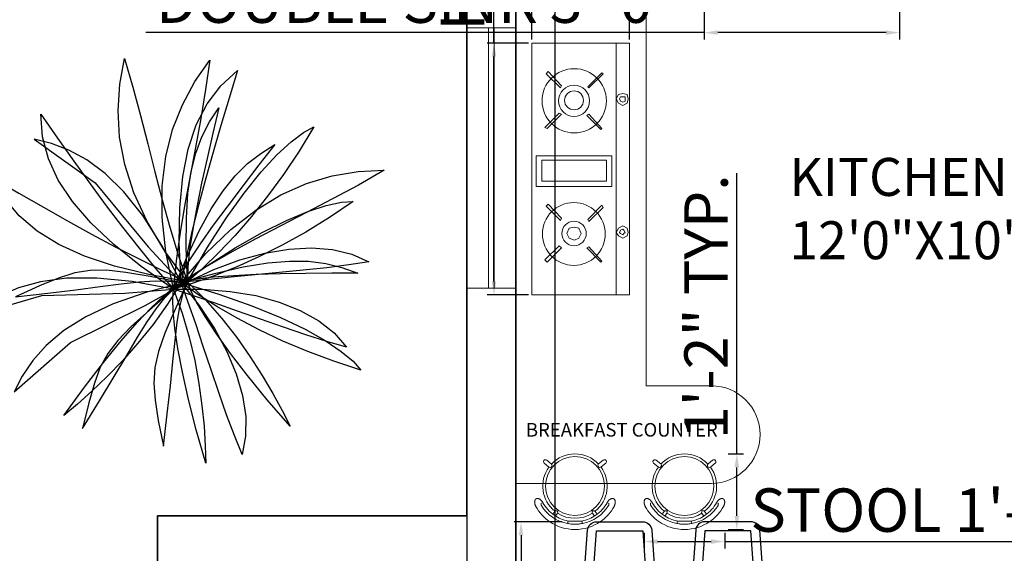
# Model space of a CAD drawing. Units: inches. Extents: x 3394 to 4794, y 965 to 1718.
# Tile 8 of 15: x 3522 to 3704, y 1450 to 1548. Entities that reach past the tile are written whole.
import ezdxf

# ---------------------------------------------------------------- set-up
doc = ezdxf.new("R2010")
doc.units = ezdxf.units.IN
for name, color, linetype, lineweight in [('A-ANNO-DIMS', 2, 'Continuous', 13), ('A-ANNO-TEXT', 7, 'Continuous', 18), ('A-AREA-IDEN', 7, 'Continuous', 18), ('A-EQPM', 8, 'Continuous', 18), ('A-FLOR-CASE', 8, 'Continuous', 18), ('A-GLAZ', 4, 'Continuous', 18), ('A-WALL', 7, 'Continuous', 35), ('CAY', 94, 'Continuous', 13), ('NOITHAT', 21, 'Continuous', 18)]:
    doc.layers.add(name, color=color, linetype=linetype, lineweight=lineweight)
doc.layers.add('DIENHOA', color=3, linetype='Continuous')
doc.layers.add('NOI THAT', color=42, linetype='Continuous')
doc.styles.get("Standard").update_dxf_attribs({"font": 'arial.ttf'})
doc.dimstyles.new('ISO-25', dxfattribs={"dimtxt": 8, "dimasz": 2.5, "dimexe": 1.25, "dimexo": 0.625, "dimtad": 1, "dimlunit": 3, "dimtxsty": 'Standard', "dimcen": 2.5, "dimadec": 0, "dimazin": 0, "dimtfac": 1, "dimtmove": 0, "dimatfit": 3, "dimfxl": 1, "dimarcsym": 0})

# ---------------------------------------------------------------- blocks, each defined once
blk = doc.blocks.new('gas 1')
for points in [[(35.93, -1.87), (35.93, 0), (0, 0), (0, -1.87)], [(8.12, -0.94), (8.44, -1.56), (8.91, -1.87), (9.53, -1.56), (9.84, -0.94), (9.53, -0.31), (8.91, -0.16), (8.44, -0.31)], [(8.59, -0.94), (8.75, -1.25), (8.91, -1.41), (9.22, -1.25), (9.37, -0.94), (9.22, -0.78), (8.91, -0.62), (8.75, -0.78)], [(27.03, -0.94), (27.34, -1.56), (27.97, -1.87), (28.59, -1.56), (28.75, -0.94), (28.59, -0.31), (27.97, -0.16), (27.34, -0.31)], [(27.5, -0.94), (27.65, -1.25), (27.97, -1.41), (28.28, -1.25), (28.28, -0.94), (28.28, -0.62), (27.97, -0.62), (27.65, -0.62)], [(19.84, -13.28), (15.47, -13.28), (15.47, -2.5), (19.84, -2.5)], [(4.84, -3.91), (4.69, -4.06), (6.72, -6.09), (6.87, -5.78)], [(12.81, -3.91), (12.5, -3.75), (10.47, -5.78), (10.78, -5.94)], [(19.22, -12.5), (16.25, -12.5), (16.25, -3.28), (19.22, -3.28)], [(23.75, -3.91), (23.59, -4.06), (25.62, -6.09), (25.78, -5.78)], [(31.71, -3.91), (31.56, -3.75), (29.53, -5.78), (29.68, -5.94)], [(7.81, -7.81), (8.12, -8.59), (8.75, -8.91), (9.53, -8.59), (9.69, -7.81), (9.53, -7.19), (8.75, -6.87), (8.12, -7.19)], [(7.03, -10), (6.72, -9.69), (4.69, -11.72), (5, -12.03)], [(12.97, -11.56), (10.94, -9.69), (10.62, -9.84), (12.65, -11.87)], [(23.75, -11.72), (23.9, -12.03), (25.93, -10), (25.78, -9.69)], [(31.87, -11.56), (29.84, -9.69), (29.53, -9.84), (31.56, -11.87)]]:
    blk.add_lwpolyline(points, close=True)
blk.add_lwpolyline([(35.93, -1.87), (35.93, -13.9), (0, -13.9), (0, -1.87)])
for centre, radius in [((8.7, -7.92), 4.48), ((27.7, -7.86), 4.58), ((8.77, -7.89), 1.74), ((27.69, -7.89), 2.22), ((27.76, -7.89), 1.35)]:
    blk.add_circle(centre, radius)
blk = doc.blocks.new('A$C02103572')
at = {"layer": 'NOI THAT'}
for p, q in [((450, 1200), (450, 0)), ((1200, 1200), (450, 1200)), ((1200, 0), (1200, 1200)), ((350, 750.1), (350, 1049.9)), ((1300, 750.1), (1300, 1049.9)), ((350, 449.9), (350, 150.1)), ((1300, 449.9), (1300, 150.1)), ((450, 0), (1200, 0))]:
    blk.add_line(p, q, dxfattribs=at)
for points in [[(350, 1100), (46.9, 1077.9, 0.396047), (0, 1028), (0, 772, 0.396047), (46.9, 722.1), (346.4, 700.3)], [(1300, 1100), (1603.1, 1077.9, -0.396047), (1650, 1028), (1650, 772, -0.396047), (1603.1, 722.1), (1303.6, 700.3)], [(350, 100), (46.9, 122.1, -0.396047), (0, 172), (0, 428, -0.396047), (46.9, 477.9), (346.4, 499.7)], [(1300, 100), (1603.1, 122.1, 0.396047), (1650, 172), (1650, 428, 0.396047), (1603.1, 477.9), (1303.6, 499.7)]]:
    blk.add_lwpolyline(points, format="xyb", dxfattribs=at)
for points in [[(353.6, 1050.1), (50, 1028), (50, 772), (350, 750.1)], [(1296.4, 1050.1), (1600, 1028), (1600, 772), (1300, 750.1)], [(353.6, 149.9), (50, 172), (50, 428), (350, 449.9)], [(1296.4, 149.9), (1600, 172), (1600, 428), (1300, 449.9)]]:
    blk.add_lwpolyline(points, dxfattribs=at)
for centre, start, end in [((351.8, 1075.1), 274.1643, 94.1643), ((1298.2, 1075.1), 85.8357, 265.8357), ((348.2, 725.2), 265.8357, 85.8357), ((1301.8, 725.2), 94.1643, 274.1643), ((348.2, 474.8), 274.1643, 94.1643), ((1301.8, 474.8), 85.8357, 265.8357), ((351.8, 124.9), 265.8357, 85.8357), ((1298.2, 124.9), 94.1643, 274.1643)]:
    blk.add_arc(centre, 25, start, end, dxfattribs=at)
blk = doc.blocks.new('SILLA 01')
for p, q in [((-0.1216, 0.2388), (-0.1198, 0.2397)), ((-0.1198, 0.2397), (-0.118, 0.2405)), ((-0.118, 0.2405), (-0.1161, 0.2412)), ((-0.1161, 0.2412), (-0.1143, 0.2419)), ((-0.1143, 0.2419), (-0.1124, 0.2426)), ((-0.1124, 0.2426), (-0.1104, 0.2431)), ((-0.1104, 0.2431), (-0.1085, 0.2437)), ((-0.1085, 0.2437), (-0.1069, 0.244)), ((-0.1069, 0.244), (-0.1053, 0.2444)), ((-0.1053, 0.2444), (-0.1037, 0.2446)), ((-0.1037, 0.2446), (-0.102, 0.2448)), ((-0.102, 0.2448), (-0.1004, 0.2449)), ((-0.1004, 0.2449), (-0.0987, 0.245)), ((-0.0987, 0.245), (-0.0971, 0.245)), ((-0.0971, 0.245), (-0.0954, 0.2449)), ((-0.0954, 0.2449), (-0.0939, 0.2448)), ((-0.0939, 0.2448), (-0.0924, 0.2446)), ((-0.0924, 0.2446), (-0.0908, 0.2443)), ((-0.0908, 0.2443), (-0.0893, 0.2439)), ((-0.0893, 0.2439), (-0.0878, 0.2435)), ((-0.0878, 0.2435), (-0.0864, 0.243)), ((-0.0864, 0.243), (-0.0849, 0.2423)), ((-0.0849, 0.2423), (-0.0836, 0.2417)), ((-0.0836, 0.2417), (-0.0826, 0.2411)), ((-0.0826, 0.2411), (-0.0817, 0.2405)), ((-0.0817, 0.2405), (-0.0808, 0.2398)), ((-0.0808, 0.2398), (-0.08, 0.239)), ((-0.1968, 0.1793), (-0.186, 0.1909)), ((-0.186, 0.1909), (-0.1746, 0.2017)), ((-0.1746, 0.2017), (-0.1626, 0.2119)), ((-0.1626, 0.2119), (-0.1501, 0.2213)), ((-0.1571, 0.1744), (-0.1381, 0.1904)), ((-0.1501, 0.2213), (-0.137, 0.23)), ((-0.1381, 0.1904), (-0.1176, 0.2043)), ((-0.137, 0.23), (-0.1234, 0.2379)), ((-0.1334, 0.1739), (-0.123, 0.1816)), ((-0.1234, 0.2379), (-0.1216, 0.2388)), ((-0.123, 0.1816), (-0.1123, 0.1887)), ((-0.1176, 0.2043), (-0.1159, 0.2052)), ((-0.1159, 0.2052), (-0.1142, 0.2058)), ((-0.1142, 0.2058), (-0.1123, 0.2062)), ((-0.1123, 0.2062), (-0.1104, 0.2063)), ((-0.1123, 0.1887), (-0.1012, 0.1952)), ((-0.1104, 0.2063), (-0.1086, 0.2062)), ((-0.1086, 0.2062), (-0.1067, 0.2058)), ((-0.1067, 0.2058), (-0.105, 0.2051)), ((-0.105, 0.2051), (-0.1033, 0.2042)), ((-0.0994, 0.1962), (-0.1012, 0.1952)), ((-0.0977, 0.1972), (-0.0994, 0.1962)), ((-0.096, 0.1983), (-0.0977, 0.1972)), ((-0.0943, 0.1994), (-0.096, 0.1983)), ((-0.0927, 0.2006), (-0.0943, 0.1994)), ((-0.0911, 0.2019), (-0.0927, 0.2006)), ((-0.0896, 0.2031), (-0.0911, 0.2019)), ((-0.0881, 0.2045), (-0.0896, 0.2031)), ((-0.0869, 0.2056), (-0.0881, 0.2045)), ((-0.0857, 0.2068), (-0.0869, 0.2056)), ((-0.0846, 0.208), (-0.0857, 0.2068)), ((-0.0835, 0.2093), (-0.0846, 0.208)), ((-0.0825, 0.2106), (-0.0835, 0.2093)), ((-0.0815, 0.212), (-0.0825, 0.2106)), ((-0.0806, 0.2133), (-0.0815, 0.212)), ((-0.0797, 0.2148), (-0.0806, 0.2133)), ((-0.08, 0.239), (-0.0792, 0.2382)), ((-0.0789, 0.2161), (-0.0797, 0.2148)), ((-0.0792, 0.2382), (-0.0785, 0.2373)), ((-0.0782, 0.2176), (-0.0789, 0.2161)), ((-0.0785, 0.2373), (-0.0779, 0.2364)), ((-0.0776, 0.219), (-0.0782, 0.2176)), ((-0.0779, 0.2364), (-0.0773, 0.2354)), ((-0.0771, 0.2205), (-0.0776, 0.219)), ((-0.0773, 0.2354), (-0.0769, 0.2344)), ((-0.0766, 0.222), (-0.0771, 0.2205)), ((-0.0769, 0.2344), (-0.0764, 0.2333)), ((-0.0762, 0.2235), (-0.0766, 0.222)), ((-0.0764, 0.2333), (-0.0761, 0.2322)), ((-0.0759, 0.2251), (-0.0762, 0.2235)), ((-0.0761, 0.2322), (-0.0759, 0.2311)), ((-0.0759, 0.2311), (-0.0757, 0.23)), ((-0.0757, 0.2266), (-0.0759, 0.2251)), ((-0.0757, 0.23), (-0.0756, 0.2289)), ((-0.0756, 0.2278), (-0.0757, 0.2266)), ((-0.0756, 0.2289), (-0.0756, 0.2278)), ((0.1165, 0.1601), (0.1387, 0.1871)), ((0.1387, 0.1871), (0.1425, 0.1901)), ((0.1425, 0.1901), (0.1471, 0.1915)), ((0.1471, 0.1915), (0.1519, 0.191)), ((0.1519, 0.191), (0.1561, 0.1886)), ((0.1561, 0.1886), (0.1592, 0.1848)), ((0.1592, 0.1848), (0.1605, 0.1801)), ((0.1605, 0.1801), (0.16, 0.1752)), ((-0.2367, 0.1191), (-0.2271, 0.1372)), ((-0.2271, 0.1372), (-0.2162, 0.1544)), ((-0.2162, 0.1544), (-0.2068, 0.1672)), ((-0.2068, 0.1672), (-0.1968, 0.1793)), ((-0.2028, 0.1156), (-0.1896, 0.1368)), ((-0.1896, 0.1368), (-0.1744, 0.1565)), ((-0.1835, 0.1171), (-0.1773, 0.1267)), ((-0.1773, 0.1267), (-0.1696, 0.1372)), ((-0.1744, 0.1565), (-0.1571, 0.1744)), ((-0.1538, 0.1223), (-0.1714, 0.1348)), ((-0.1696, 0.1372), (-0.1614, 0.1472)), ((-0.1614, 0.1472), (-0.1525, 0.1566)), ((-0.1538, 0.1223), (-0.1511, 0.1194)), ((-0.1525, 0.1566), (-0.1432, 0.1655)), ((-0.1432, 0.1655), (-0.1334, 0.1739)), ((0.1136, 0.1509), (0.1141, 0.1558)), ((0.115, 0.1462), (0.1136, 0.1509)), ((0.1141, 0.1558), (0.1165, 0.1601)), ((0.118, 0.1423), (0.115, 0.1462)), ((0.1222, 0.14), (0.118, 0.1423)), ((0.127, 0.1394), (0.1222, 0.14)), ((0.1317, 0.1408), (0.127, 0.1394)), ((0.1354, 0.1439), (0.1317, 0.1408)), ((0.1577, 0.1709), (0.1354, 0.1439)), ((0.16, 0.1752), (0.1577, 0.1709)), ((-0.2609, 0.041), (-0.2571, 0.0611)), ((-0.2571, 0.0611), (-0.2518, 0.081)), ((-0.2518, 0.081), (-0.245, 0.1003)), ((-0.245, 0.1003), (-0.2367, 0.1191)), ((-0.2281, 0.0453), (-0.2221, 0.0696)), ((-0.2221, 0.0696), (-0.2136, 0.0931)), ((-0.2136, 0.0931), (-0.2028, 0.1156)), ((-0.2101, 0.0535), (-0.207, 0.0646)), ((-0.207, 0.0646), (-0.2034, 0.0756)), ((-0.2034, 0.0756), (-0.1993, 0.0864)), ((-0.1993, 0.0864), (-0.1945, 0.0969)), ((-0.1945, 0.0969), (-0.1893, 0.1071)), ((-0.1893, 0.1071), (-0.1835, 0.1171)), ((-0.1828, 0.1184), (-0.1651, 0.1058)), ((-0.1616, 0.1042), (-0.1651, 0.1058)), ((-0.1577, 0.1041), (-0.1616, 0.1042)), ((-0.1541, 0.1055), (-0.1577, 0.1041)), ((-0.1513, 0.1083), (-0.1541, 0.1055)), ((-0.1498, 0.1118), (-0.1513, 0.1083)), ((-0.1511, 0.1194), (-0.1497, 0.1158)), ((-0.1497, 0.1158), (-0.1498, 0.1118)), ((-0.264, 0), (-0.2632, 0.0205)), ((-0.2632, -0.0205), (-0.264, 0)), ((-0.2632, 0.0205), (-0.2609, 0.041)), ((-0.2318, 0), (-0.2317, 0.0057)), ((-0.2317, -0.0057), (-0.2318, 0)), ((-0.2317, 0.0057), (-0.2315, 0.0114)), ((-0.2315, 0.0114), (-0.2312, 0.017)), ((-0.2312, 0.017), (-0.2307, 0.0227)), ((-0.2307, 0.0227), (-0.2301, 0.0283)), ((-0.2301, 0.0283), (-0.2294, 0.034)), ((-0.2294, 0.034), (-0.2285, 0.0396)), ((-0.2285, 0.0396), (-0.2275, 0.0452)), ((-0.2125, 0.0422), (-0.2275, 0.0452)), ((-0.2125, 0.0422), (-0.2101, 0.0535)), ((-0.2125, 0.0422), (-0.2125, -0.0422)), ((-0.2609, -0.041), (-0.2632, -0.0205)), ((-0.2571, -0.0611), (-0.2609, -0.041)), ((-0.2315, -0.0114), (-0.2317, -0.0057)), ((-0.2312, -0.017), (-0.2315, -0.0114)), ((-0.2307, -0.0227), (-0.2312, -0.017)), ((-0.2301, -0.0283), (-0.2307, -0.0227)), ((-0.2294, -0.034), (-0.2301, -0.0283)), ((-0.2285, -0.0396), (-0.2294, -0.034)), ((-0.2275, -0.0452), (-0.2285, -0.0396)), ((-0.2221, -0.0696), (-0.2281, -0.0453)), ((-0.2125, -0.0422), (-0.2275, -0.0452)), ((-0.2101, -0.0535), (-0.2125, -0.0422)), ((-0.207, -0.0646), (-0.2101, -0.0535)), ((-0.2518, -0.081), (-0.2571, -0.0611)), ((-0.245, -0.1003), (-0.2518, -0.081)), ((-0.2367, -0.1191), (-0.245, -0.1003)), ((-0.2271, -0.1372), (-0.2367, -0.1191)), ((-0.2136, -0.0931), (-0.2221, -0.0696)), ((-0.2028, -0.1156), (-0.2136, -0.0931)), ((-0.2034, -0.0756), (-0.207, -0.0646)), ((-0.1993, -0.0864), (-0.2034, -0.0756)), ((-0.1896, -0.1368), (-0.2028, -0.1156)), ((-0.1945, -0.0969), (-0.1993, -0.0864)), ((-0.1893, -0.1071), (-0.1945, -0.0969)), ((-0.1835, -0.1171), (-0.1893, -0.1071)), ((-0.1773, -0.1267), (-0.1835, -0.1171)), ((-0.1828, -0.1184), (-0.1651, -0.1058)), ((-0.1651, -0.1058), (-0.1616, -0.1042)), ((-0.1616, -0.1042), (-0.1577, -0.1041)), ((-0.1577, -0.1041), (-0.1541, -0.1055)), ((-0.1541, -0.1055), (-0.1513, -0.1083)), ((-0.1511, -0.1194), (-0.1538, -0.1223)), ((-0.1513, -0.1083), (-0.1498, -0.1118)), ((-0.1497, -0.1158), (-0.1511, -0.1194)), ((-0.1498, -0.1118), (-0.1497, -0.1158)), ((-0.2162, -0.1544), (-0.2271, -0.1372)), ((-0.2068, -0.1672), (-0.2162, -0.1544)), ((-0.1968, -0.1793), (-0.2068, -0.1672)), ((-0.186, -0.1909), (-0.1968, -0.1793)), ((-0.1744, -0.1565), (-0.1896, -0.1368)), ((-0.1696, -0.1372), (-0.1773, -0.1267)), ((-0.1571, -0.1744), (-0.1744, -0.1565)), ((-0.1538, -0.1223), (-0.1714, -0.1348)), ((-0.1614, -0.1472), (-0.1696, -0.1372)), ((-0.1525, -0.1566), (-0.1614, -0.1472)), ((-0.1381, -0.1904), (-0.1571, -0.1744)), ((-0.1432, -0.1655), (-0.1525, -0.1566)), ((-0.1334, -0.1739), (-0.1432, -0.1655)), ((-0.123, -0.1816), (-0.1334, -0.1739)), ((0.1136, -0.1509), (0.115, -0.1462)), ((0.1141, -0.1558), (0.1136, -0.1509)), ((0.1165, -0.1601), (0.1141, -0.1558)), ((0.115, -0.1462), (0.118, -0.1423)), ((0.1165, -0.1601), (0.1387, -0.1871)), ((0.118, -0.1423), (0.1222, -0.14)), ((0.1222, -0.14), (0.127, -0.1394)), ((0.127, -0.1394), (0.1317, -0.1408)), ((0.1317, -0.1408), (0.1354, -0.1439)), ((0.1577, -0.1709), (0.1354, -0.1439)), ((0.1577, -0.1709), (0.16, -0.1752)), ((0.16, -0.1752), (0.1605, -0.1801)), ((-0.1746, -0.2017), (-0.186, -0.1909)), ((-0.1626, -0.2119), (-0.1746, -0.2017)), ((-0.1501, -0.2213), (-0.1626, -0.2119)), ((-0.137, -0.23), (-0.1501, -0.2213)), ((-0.1176, -0.2043), (-0.1381, -0.1904)), ((-0.1234, -0.2379), (-0.137, -0.23)), ((-0.1216, -0.2388), (-0.1234, -0.2379)), ((-0.1123, -0.1887), (-0.123, -0.1816)), ((-0.1198, -0.2397), (-0.1216, -0.2388)), ((-0.1159, -0.2052), (-0.1176, -0.2043)), ((-0.1142, -0.2058), (-0.1159, -0.2052)), ((-0.1123, -0.2062), (-0.1142, -0.2058)), ((-0.1012, -0.1952), (-0.1123, -0.1887)), ((-0.1104, -0.2063), (-0.1123, -0.2062)), ((-0.1086, -0.2062), (-0.1104, -0.2063)), ((-0.1067, -0.2058), (-0.1086, -0.2062)), ((-0.105, -0.2051), (-0.1067, -0.2058)), ((-0.1033, -0.2042), (-0.105, -0.2051)), ((-0.1012, -0.1952), (-0.0994, -0.1962)), ((-0.0994, -0.1962), (-0.0977, -0.1972)), ((-0.0977, -0.1972), (-0.096, -0.1983)), ((-0.096, -0.1983), (-0.0943, -0.1994)), ((-0.0943, -0.1994), (-0.0927, -0.2006)), ((-0.0927, -0.2006), (-0.0911, -0.2019)), ((-0.0911, -0.2019), (-0.0896, -0.2031)), ((-0.0896, -0.2031), (-0.0881, -0.2045)), ((-0.0881, -0.2045), (-0.0869, -0.2056)), ((-0.0869, -0.2056), (-0.0857, -0.2068)), ((-0.0857, -0.2068), (-0.0846, -0.208)), ((-0.0846, -0.208), (-0.0835, -0.2093)), ((-0.0835, -0.2093), (-0.0825, -0.2106)), ((-0.0825, -0.2106), (-0.0815, -0.212)), ((-0.0815, -0.212), (-0.0806, -0.2133)), ((-0.08, -0.239), (-0.0808, -0.2398)), ((-0.0806, -0.2133), (-0.0797, -0.2148)), ((-0.0792, -0.2382), (-0.08, -0.239)), ((-0.0797, -0.2148), (-0.0789, -0.2161)), ((-0.0785, -0.2373), (-0.0792, -0.2382)), ((-0.0789, -0.2161), (-0.0782, -0.2176)), ((-0.0779, -0.2364), (-0.0785, -0.2373)), ((-0.0782, -0.2176), (-0.0776, -0.219)), ((-0.0773, -0.2354), (-0.0779, -0.2364)), ((-0.0776, -0.219), (-0.0771, -0.2205)), ((-0.0769, -0.2344), (-0.0773, -0.2354)), ((-0.0771, -0.2205), (-0.0766, -0.222)), ((-0.0764, -0.2333), (-0.0769, -0.2344)), ((-0.0766, -0.222), (-0.0762, -0.2235)), ((-0.0761, -0.2322), (-0.0764, -0.2333)), ((-0.0762, -0.2235), (-0.0759, -0.2251)), ((-0.0759, -0.2311), (-0.0761, -0.2322)), ((-0.0759, -0.2251), (-0.0757, -0.2266)), ((-0.0757, -0.23), (-0.0759, -0.2311)), ((-0.0757, -0.2266), (-0.0756, -0.2278)), ((-0.0756, -0.2289), (-0.0757, -0.23)), ((-0.0756, -0.2278), (-0.0756, -0.2289)), ((0.1425, -0.1901), (0.1387, -0.1871)), ((0.1471, -0.1915), (0.1425, -0.1901)), ((0.1519, -0.191), (0.1471, -0.1915)), ((0.1561, -0.1886), (0.1519, -0.191)), ((0.1592, -0.1848), (0.1561, -0.1886)), ((0.1605, -0.1801), (0.1592, -0.1848)), ((-0.118, -0.2405), (-0.1198, -0.2397)), ((-0.1161, -0.2412), (-0.118, -0.2405)), ((-0.1143, -0.2419), (-0.1161, -0.2412)), ((-0.1124, -0.2426), (-0.1143, -0.2419)), ((-0.1104, -0.2431), (-0.1124, -0.2426)), ((-0.1085, -0.2437), (-0.1104, -0.2431)), ((-0.1069, -0.244), (-0.1085, -0.2437)), ((-0.1053, -0.2444), (-0.1069, -0.244)), ((-0.1037, -0.2446), (-0.1053, -0.2444)), ((-0.102, -0.2448), (-0.1037, -0.2446)), ((-0.1004, -0.2449), (-0.102, -0.2448)), ((-0.0987, -0.245), (-0.1004, -0.2449)), ((-0.0971, -0.245), (-0.0987, -0.245)), ((-0.0954, -0.2449), (-0.0971, -0.245)), ((-0.0939, -0.2448), (-0.0954, -0.2449)), ((-0.0924, -0.2446), (-0.0939, -0.2448)), ((-0.0908, -0.2443), (-0.0924, -0.2446)), ((-0.0893, -0.2439), (-0.0908, -0.2443)), ((-0.0878, -0.2435), (-0.0893, -0.2439)), ((-0.0864, -0.243), (-0.0878, -0.2435)), ((-0.0849, -0.2423), (-0.0864, -0.243)), ((-0.0836, -0.2417), (-0.0849, -0.2423)), ((-0.0826, -0.2411), (-0.0836, -0.2417)), ((-0.0817, -0.2405), (-0.0826, -0.2411)), ((-0.0808, -0.2398), (-0.0817, -0.2405))]:
    blk.add_line(p, q)
blk.add_circle((0, 0), 0.1793)
for start, end in [(53.88178, 141.5278), (313.19891, 46.80109), (147.34891, 212.65109), (218.4722, 306.11822)]:
    blk.add_arc((0, 0), 0.196, start, end)
blk = doc.blocks.new('Cay03_mb')
at = {"layer": 'DIENHOA'}
for p, q in [((118.6, 555.3), (166.2, 599.1)), ((166.2, 599.1), (142.2, 519.4)), ((79.5, 503.7), (118.6, 555.3)), ((142.2, 519.4), (119, 441.7)), ((48.6, 443.6), (79.5, 503.7)), ((25.5, 374.3), (48.6, 443.6)), ((119, 441.7), (96.7, 365.6)), ((-365.2, 390.3), (-414.4, 402.8)), ((-414.4, 402.8), (-240.2, 277.8)), ((-314.9, 371.3), (-365.2, 390.3)), ((-263.5, 343.5), (-314.9, 371.3)), ((9.9, 295.3), (25.5, 374.3)), ((-211.2, 304.6), (-263.5, 343.5)), ((96.7, 365.6), (75.6, 290.6)), ((436.8, 297.2), (511, 309.6)), ((511, 309.6), (585.9, 313.5)), ((585.9, 313.5), (511.8, 271.4)), ((-158, 252.3), (-211.2, 304.6)), ((1.6, 205.7), (9.9, 295.3)), ((75.6, 290.6), (55.7, 216.3)), ((363.4, 275.4), (436.8, 297.2)), ((-240.2, 277.8), (-88.4, 94.9)), ((290.6, 243.2), (363.4, 275.4)), ((511.8, 271.4), (437.6, 231.5)), ((-104.2, 184.4), (-158, 252.3)), ((218.5, 199.8), (290.6, 243.2)), ((437.6, 231.5), (363.7, 192.9)), ((0.2, 104.9), (1.6, 205.7)), ((55.7, 216.3), (37.3, 142.1)), ((147, 144.1), (218.5, 199.8)), ((-49.6, 98.5), (-104.2, 184.4)), ((363.7, 192.9), (290.2, 154.9)), ((37.3, 142.1), (20.5, 67.6)), ((75.9, 75.2), (147, 144.1)), ((290.2, 154.9), (217.4, 116.6)), ((217.4, 116.6), (145.5, 77.3)), ((-88.4, 94.9), (5.4, -7.8)), ((5.4, -7.8), (-49.6, 98.5)), ((5.4, -7.8), (0.2, 104.9)), ((5.4, -7.8), (75.9, 75.2)), ((20.5, 67.6), (5.4, -7.8)), ((145.5, 77.3), (74.7, 36.1)), ((74.7, 36.1), (5.4, -7.8)), ((100.3, 18.4), (182.2, 37.2)), ((182.2, 37.2), (253, 48.9)), ((253, 48.9), (314.6, 54.1)), ((314.6, 54.1), (369.2, 53.3)), ((369.2, 53.3), (418.6, 46.8)), ((418.6, 46.8), (464.9, 35.2)), ((464.9, 35.2), (510, 19)), ((-345, 5.4), (-399.6, -17.1)), ((-298.6, 20.1), (-345, 5.4)), ((-254.7, 27.4), (-298.6, 20.1)), ((-208, 27.8), (-254.7, 27.4)), ((-152.7, 21.7), (-208, 27.8)), ((-83.4, 9.7), (-152.7, 21.7)), ((5.4, -7.8), (-83.4, 9.7)), ((5.4, -7.8), (100.3, 18.4)), ((46.3, 0.9), (5.4, -7.8)), ((96.7, 7.5), (46.3, 0.9)), ((155, 12.2), (96.7, 7.5)), ((219.6, 15.4), (155, 12.2)), ((289, 17.4), (219.6, 15.4)), ((361.6, 18.5), (289, 17.4)), ((435.8, 18.9), (361.6, 18.5)), ((510, 19), (435.8, 18.9)), ((-399.6, -17.1), (-468, -47.9)), ((-375.6, -37.8), (-295.3, -27.9)), ((-295.3, -27.9), (-225.8, -18.9)), ((-225.8, -18.9), (-165.8, -11.3)), ((-165.8, -11.3), (-114, -5.7)), ((-114, -5.7), (-69, -2.9)), ((-69, -2.9), (-29.6, -3.4)), ((-45.1, -46.3), (-16.5, -22.4)), ((5.4, -7.8), (-33.2, -69.5)), ((-29.6, -3.4), (5.4, -7.8)), ((-16.5, -22.4), (5.4, -7.8)), ((5.4, -7.8), (56.8, -73.3)), ((25.9, -64.4), (5.4, -7.8)), ((5.4, -7.8), (112.8, -40.3)), ((53.5, -41.6), (5.4, -7.8)), ((-468, -47.9), (-375.6, -37.8)), ((-79.8, -79.6), (-45.1, -46.3)), ((107, -75.7), (53.5, -41.6)), ((112.8, -40.3), (207.5, -73.8)), ((-120.2, -122.1), (-79.8, -79.6)), ((-33.2, -69.5), (-74.6, -127.3)), ((47, -125.9), (25.9, -64.4)), ((56.8, -73.3), (100.4, -139.1)), ((165.5, -109.6), (107, -75.7)), ((207.5, -73.8), (289.5, -107.6)), ((228.7, -142.8), (165.5, -109.6)), ((289.5, -107.6), (359.3, -141.1)), ((-165.9, -174.1), (-120.2, -122.1)), ((-74.6, -127.3), (-117.8, -181.1)), ((68.7, -190.6), (47, -125.9)), ((100.4, -139.1), (135.9, -204.3)), ((296, -174.7), (228.7, -142.8)), ((359.3, -141.1), (416.9, -173.5)), ((-216.3, -235.6), (-165.9, -174.1)), ((-117.8, -181.1), (-162.1, -230.9)), ((90.8, -256.6), (68.7, -190.6)), ((367.1, -204.8), (296, -174.7)), ((416.9, -173.5), (462.6, -204.2)), ((135.9, -204.3), (162.8, -268.3)), ((441.6, -232.7), (367.1, -204.8)), ((462.6, -204.2), (496.5, -232.5)), ((-271, -306.6), (-216.3, -235.6)), ((-162.1, -230.9), (-206.3, -276.5)), ((518.9, -257.7), (441.6, -232.7)), ((496.5, -232.5), (518.9, -257.7)), ((-206.3, -276.5), (-249.6, -317.8)), ((113.1, -322.2), (90.8, -256.6)), ((162.8, -268.3), (181, -330.4)), ((-329.5, -387.1), (-271, -306.6)), ((-249.6, -317.8), (-291, -354.7)), ((135.4, -385.6), (113.1, -322.2)), ((181, -330.4), (190, -390)), ((-291, -354.7), (-329.5, -387.1)), ((157.6, -445), (135.4, -385.6)), ((190, -390), (189.6, -446.3)), ((179.5, -498.7), (157.6, -445)), ((189.6, -446.3), (179.5, -498.7))]:
    blk.add_line(p, q, dxfattribs=at)
for points in [[(23.7, -5.4), (-41, 82.2), (-91.8, 167.1), (-129.7, 249.5), (-155.6, 329.6), (-170.2, 407.8), (-174.7, 484.2), (-169.8, 559.3), (-156.5, 633.1)], [(-156.5, 633.1), (-132.5, 551.3), (-110.5, 470), (-89.8, 389.2), (-69.6, 309), (-49, 229.4), (-27.1, 150.4), (-3.2, 72.1), (23.7, -5.4)], [(-16.4, -26.7), (-38.3, 80), (-48.9, 178.3), (-48.7, 269), (-38.5, 352.6), (-19.1, 429.7), (9, 501), (44.9, 567.1), (87.9, 628.5)], [(87.9, 628.5), (75.5, 544.2), (61.3, 461.2), (46.1, 379.1), (30.8, 297.8), (16.1, 216.9), (2.9, 136), (-8.3, 54.9), (-16.4, -26.7)], [(23.7, -5.4), (19.8, 93), (20.3, 177), (25, 248.5), (34, 309.8), (47.3, 362.7), (64.9, 409.3), (86.8, 451.7), (112.9, 491.9)], [(112.9, 491.9), (96, 419.7), (79.5, 347.4), (63.9, 276.5), (50, 208.4), (38.4, 144.8), (29.7, 86.9), (24.6, 36.3), (23.7, -5.4)], [(-395.6, 473.7), (-347.5, 405.6), (-300.6, 339.5), (-254.3, 275.1), (-208.3, 212.3), (-161.9, 150.9), (-114.8, 90.7), (-66.5, 31.6), (-16.4, -26.7)], [(-16.4, -26.7), (-108.3, 38.6), (-186.9, 101.7), (-252.4, 163.5), (-305.1, 224.4), (-345.4, 285.2), (-373.7, 346.6), (-390.4, 409.2), (-395.6, 473.7)], [(384.3, 437.5), (342.2, 367.8), (298.1, 301.7), (252.6, 239.4), (206.1, 181.1), (159.4, 127.2), (113, 78), (67.6, 33.6), (23.7, -5.4)], [(23.7, -5.4), (79.9, 91.7), (134.1, 176.2), (185.8, 248.4), (234.3, 308.7), (279, 357.3), (319.3, 394.8), (354.6, 421.4), (384.3, 437.5)], [(273.2, 387.3), (227.6, 328.8), (182.3, 270.1), (138.4, 212.3), (97.2, 156.4), (60, 103.4), (27.8, 54.6), (1.9, 10.8), (-16.4, -26.7)], [(-16.4, -26.7), (21.4, 64.2), (57, 140.3), (91.4, 203.3), (125.2, 255.1), (159.5, 297.5), (195, 332.5), (232.7, 361.8), (273.2, 387.3)], [(-530.5, 289.7), (-458.3, 248.1), (-387.9, 207.8), (-318.9, 168.7), (-250.8, 131.1), (-182.9, 94.8), (-114.9, 59.9), (-46.2, 26.5), (23.7, -5.4)], [(23.7, -5.4), (-87.2, 15.2), (-185, 39.6), (-270.3, 68.2), (-343.7, 101.4), (-405.9, 139.7), (-457.3, 183.5), (-498.7, 233.4), (-530.5, 289.7)], [(496.7, 224), (429.4, 178.4), (361.6, 136.9), (294.1, 99.5), (227.5, 66.1), (162.4, 36.7), (99.7, 11.5), (39.8, -9.7), (-16.4, -26.7)], [(-16.4, -26.7), (75.4, 37.9), (160.1, 91.8), (237.3, 135.7), (306.6, 170), (367.6, 195.4), (419.9, 212.5), (463.1, 221.9), (496.7, 224)], [(23.7, -5.4), (99.3, 29.7), (173.2, 57.1), (244.8, 76.7), (313.3, 88.3), (377.9, 91.8), (437.9, 87), (492.7, 73.8), (541.4, 52)], [(541.4, 52), (484.1, 42.9), (421.2, 34.8), (354.4, 27.6), (285.4, 20.9), (216.1, 14.5), (148.2, 8.1), (83.5, 1.6), (23.7, -5.4)], [(-16.4, -26.7), (-134, -4.7), (-235.3, 5.3), (-322, 4.7), (-395.9, -5), (-458.7, -22.3), (-512.3, -45.7), (-558.2, -73.6), (-598.4, -104.7)], [(-598.4, -104.7), (-392.7, -44.4), (-155, -37.4), (-16.4, -26.7)], [(-471.9, -320.3), (-310.5, -179.3), (-97.7, -73.3), (23.7, -5.4)], [(23.7, -5.4), (-92.3, -34.8), (-188.4, -68.2), (-266.9, -105.1), (-329.9, -144.9), (-379.7, -187), (-418.5, -230.7), (-448.5, -275.3), (-471.9, -320.3)], [(-276.2, -424.4), (-227.3, -345.4), (-185.7, -276.1), (-150, -215.7), (-119.1, -163.8), (-91.5, -119.5), (-66, -82.3), (-41.4, -51.6), (-16.4, -26.7)], [(-16.4, -26.7), (-84.9, -86), (-137, -133.1), (-175.8, -173), (-204.3, -210), (-225.5, -249.1), (-242.5, -294.7), (-258.4, -351.6), (-276.2, -424.4)], [(23.7, -5.4), (-13.6, -87.9), (-41.1, -152.6), (-59.6, -205), (-69.9, -250.7), (-72.8, -295), (-69.2, -343.6), (-59.7, -401.9), (-45.3, -475.5)], [(-45.3, -475.5), (-34.1, -383.2), (-25.4, -302.8), (-18.3, -233.1), (-12, -172.9), (-5.6, -121.2), (2, -76.8), (11.4, -38.5), (23.7, -5.4)], [(76.2, -524.2), (48.8, -428.5), (26.6, -341.7), (9.2, -264.1), (-3.6, -196.1), (-12.3, -138), (-17.1, -90.2), (-18.3, -53), (-16.4, -26.7)], [(-16.4, -26.7), (66.9, -26.6), (145.6, -32.7), (218.8, -44.9), (285.8, -63.1), (345.9, -87.1), (398.4, -116.6), (442.6, -151.6), (477.6, -191.8)], [(477.6, -191.8), (421.8, -176), (361.3, -156.9), (297.6, -135.5), (232.2, -112.6), (166.6, -89.4), (102.3, -66.6), (40.8, -45.4), (-16.4, -26.7)], [(-16.4, -26.7), (8.5, -95.1), (28.5, -163.3), (44.3, -230.6), (56.3, -296.1), (65, -359), (70.9, -418.5), (74.5, -473.9), (76.2, -524.2)], [(316.5, -418.1), (251.4, -342.8), (194.8, -273.3), (146.5, -210.2), (106.3, -153.8), (74.1, -104.7), (49.7, -63.4), (32.9, -30.1), (23.7, -5.4)], [(23.7, -5.4), (74.9, -57.1), (121.8, -110.6), (164.3, -165), (202.7, -219.4), (237, -272.9), (267.3, -324.5), (293.7, -373.2), (316.5, -418.1)]]:
    blk.add_lwpolyline(points, dxfattribs=at)
blk = doc.blocks.new('WIN-48IN')
for p, q in [((9, 48), (0, 48)), ((4, 0), (4, 48)), ((5, 0), (5, 48)), ((9, 0), (0, 0))]:
    blk.add_line(p, q)
blk = doc.blocks.new('*D88')
at = {"layer": 'A-ANNO-DIMS', "color": 0, "lineweight": -2, "transparency": 16777216}
for p, q in [((3637.38, 1453.56), (3637.38, 1450.71)), ((3652.23, 1453.56), (3652.23, 1450.7)), ((3639.88, 1451.96), (3649.73, 1451.96)), ((3652.23, 1451.95), (3745.7, 1451.93))]:
    blk.add_line(p, q, dxfattribs=at)
at = {"layer": 'A-ANNO-DIMS', "color": 0, "transparency": 16777216}
for points in [[(3639.88, 1452.37), (3639.88, 1451.54), (3637.38, 1451.96)], [(3649.73, 1452.37), (3649.73, 1451.54), (3652.23, 1451.95)]]:
    blk.add_solid(points, dxfattribs=at)
at = {"layer": 'Defpoints', "color": 0, "transparency": 16777216}
for p in [(3637.38, 1454.19), (3652.23, 1454.18), (3652.23, 1451.95)]:
    blk.add_point(p, dxfattribs=at)
at = {"layer": 'A-ANNO-DIMS', "color": 0, "transparency": 16777216, "insert": (3700.21, 1456.71), "char_height": 8, "attachment_point": 5, "rotation": 359.9851}
blk.add_mtext('STOOL 1\'-3" TYP.', dxfattribs=at)
blk = doc.blocks.new('*D89')
at = {"layer": 'A-ANNO-DIMS', "color": 0, "lineweight": -2, "transparency": 16777216}
for p, q in [((3654.46, 1468.13), (3654.48, 1519.89)), ((3652.86, 1468.13), (3655.71, 1468.12)), ((3654.46, 1456.68), (3654.46, 1465.63)), ((3652.86, 1454.18), (3655.71, 1454.18))]:
    blk.add_line(p, q, dxfattribs=at)
at = {"layer": 'A-ANNO-DIMS', "color": 0, "transparency": 16777216}
for points in [[(3654.05, 1465.63), (3654.88, 1465.63), (3654.46, 1468.13)], [(3654.04, 1456.68), (3654.88, 1456.68), (3654.46, 1454.18)]]:
    blk.add_solid(points, dxfattribs=at)
at = {"layer": 'Defpoints', "color": 0, "transparency": 16777216}
for p in [(3652.24, 1468.13), (3654.46, 1468.13), (3652.23, 1454.18)]:
    blk.add_point(p, dxfattribs=at)
at = {"layer": 'A-ANNO-DIMS', "color": 0, "transparency": 16777216, "insert": (3649.83, 1495.26), "char_height": 8, "attachment_point": 5, "rotation": 89.9851}
blk.add_mtext('1\'-2" TYP.', dxfattribs=at)
blk = doc.blocks.new('*D96')
at = {"layer": 'A-ANNO-DIMS', "color": 0, "lineweight": -2, "transparency": 16777216}
for p, q in [((3648.46, 1550.57), (3648.46, 1544.54)), ((3684.46, 1550.57), (3684.46, 1544.54)), ((3648.46, 1545.79), (3545.58, 1545.79)), ((3681.96, 1545.79), (3650.96, 1545.79))]:
    blk.add_line(p, q, dxfattribs=at)
at = {"layer": 'A-ANNO-DIMS', "color": 0, "transparency": 16777216}
for points in [[(3650.96, 1546.21), (3650.96, 1545.38), (3648.46, 1545.79)], [(3681.96, 1546.21), (3681.96, 1545.38), (3684.46, 1545.79)]]:
    blk.add_solid(points, dxfattribs=at)
at = {"layer": 'Defpoints', "color": 0, "transparency": 16777216}
for p in [(3648.46, 1551.19), (3684.46, 1551.19), (3648.46, 1545.79)]:
    blk.add_point(p, dxfattribs=at)
at = {"layer": 'A-ANNO-DIMS', "color": 0, "transparency": 16777216, "insert": (3595.77, 1550.56), "char_height": 8, "attachment_point": 5}
blk.add_mtext('DOUBLE SINK 3\'-0"', dxfattribs=at)
blk = doc.blocks.new('*D98')
at = {"layer": 'A-ANNO-DIMS', "color": 0, "lineweight": -2, "transparency": 16777216}
for p, q in [((3609.73, 1543.87), (3609.73, 1620.64)), ((3616.08, 1543.87), (3608.48, 1543.87)), ((3609.73, 1499.92), (3609.73, 1541.37)), ((3616.08, 1497.42), (3608.48, 1497.42))]:
    blk.add_line(p, q, dxfattribs=at)
at = {"layer": 'A-ANNO-DIMS', "color": 0, "transparency": 16777216}
for points in [[(3609.32, 1541.37), (3610.15, 1541.37), (3609.73, 1543.87)], [(3609.32, 1499.92), (3610.15, 1499.92), (3609.73, 1497.42)]]:
    blk.add_solid(points, dxfattribs=at)
at = {"layer": 'Defpoints', "color": 0, "transparency": 16777216}
for p in [(3609.73, 1543.87), (3616.7, 1543.87), (3616.7, 1497.42)]:
    blk.add_point(p, dxfattribs=at)
at = {"layer": 'A-ANNO-DIMS', "color": 0, "transparency": 16777216, "insert": (3604.97, 1583.5), "char_height": 8, "attachment_point": 5, "rotation": 90}
blk.add_mtext('HOB 3\'-10 1/2"', dxfattribs=at)
blk = doc.blocks.new('*D99')
at = {"layer": 'A-ANNO-DIMS', "color": 0, "lineweight": -2, "transparency": 16777216}
for p, q in [((3616.7, 1544.5), (3616.7, 1552.09)), ((3634.67, 1544.5), (3634.67, 1552.09)), ((3619.2, 1550.84), (3632.17, 1550.84)), ((3634.67, 1550.84), (3658.94, 1550.84))]:
    blk.add_line(p, q, dxfattribs=at)
at = {"layer": 'A-ANNO-DIMS', "color": 0, "transparency": 16777216}
for points in [[(3619.2, 1551.25), (3619.2, 1550.42), (3616.7, 1550.84)], [(3632.17, 1551.25), (3632.17, 1550.42), (3634.67, 1550.84)]]:
    blk.add_solid(points, dxfattribs=at)
at = {"layer": 'Defpoints', "color": 0, "transparency": 16777216}
for p in [(3634.67, 1550.84), (3616.7, 1543.87), (3634.67, 1543.87)]:
    blk.add_point(p, dxfattribs=at)
at = {"layer": 'A-ANNO-DIMS', "color": 0, "transparency": 16777216, "insert": (3648.06, 1555.55), "char_height": 8, "attachment_point": 5}
blk.add_mtext('1\'-6"', dxfattribs=at)
blk = doc.blocks.new('*D104')
at = {"layer": 'A-ANNO-DIMS', "color": 0, "lineweight": -2, "transparency": 16777216}
for p, q in [((3622.3, 1455.61), (3613.46, 1455.61)), ((3614.71, 1453.11), (3614.71, 1403.36)), ((3622.3, 1400.86), (3613.46, 1400.86)), ((3614.71, 1400.86), (3614.71, 1309.18))]:
    blk.add_line(p, q, dxfattribs=at)
at = {"layer": 'A-ANNO-DIMS', "color": 0, "transparency": 16777216}
for points in [[(3614.29, 1453.11), (3615.13, 1453.11), (3614.71, 1455.61)], [(3614.29, 1403.36), (3615.13, 1403.36), (3614.71, 1400.86)]]:
    blk.add_solid(points, dxfattribs=at)
at = {"layer": 'Defpoints', "color": 0, "transparency": 16777216}
for p in [(3622.92, 1455.61), (3614.71, 1400.86), (3622.92, 1400.86)]:
    blk.add_point(p, dxfattribs=at)
at = {"layer": 'A-ANNO-DIMS', "color": 0, "transparency": 16777216, "insert": (3609.95, 1353.77), "char_height": 8, "attachment_point": 5, "rotation": 90}
blk.add_mtext('DINING SET 4\'-7"', dxfattribs=at)
blk = doc.blocks.new('*D123')
at = {"layer": 'A-ANNO-DIMS', "color": 0, "lineweight": -2, "transparency": 16777216}
for p, q in [((3604.74, 1582.06), (3604.74, 987.36)), ((3620.92, 1582.06), (3620.92, 987.36)), ((3607.24, 988.61), (3618.42, 988.61)), ((3620.92, 988.61), (3645.18, 988.61))]:
    blk.add_line(p, q, dxfattribs=at)
at = {"layer": 'A-ANNO-DIMS', "color": 0, "transparency": 16777216}
for points in [[(3607.24, 989.03), (3607.24, 988.2), (3604.74, 988.61)], [(3618.42, 989.03), (3618.42, 988.2), (3620.92, 988.61)]]:
    blk.add_solid(points, dxfattribs=at)
at = {"layer": 'Defpoints', "color": 0, "transparency": 16777216}
for p in [(3604.74, 1582.68), (3620.92, 1582.68), (3620.92, 988.61)]:
    blk.add_point(p, dxfattribs=at)
at = {"layer": 'A-ANNO-DIMS', "color": 0, "transparency": 16777216, "insert": (3634.3, 993.25), "char_height": 8, "attachment_point": 5}
blk.add_mtext('1\'-4"', dxfattribs=at)

msp = doc.modelspace()

# ---------------------------------------------------------------- linework, layer by layer
at = {"layer": 'A-FLOR-CASE'}
for p, q in [((3637.745, 1549.682), (3637.745, 1480.682)), ((3637.745, 1480.682), (3649.745, 1480.682)), ((3637.745, 1480.682), (3649.745, 1480.682)), ((3613.745, 1462.682), (3649.745, 1462.682))]:
    msp.add_line(p, q, dxfattribs=at)
msp.add_arc((3649.745, 1471.682), 9, 270, 90, dxfattribs=at)
at = {"layer": 'A-WALL'}
for p, q in [((3604.745, 1636.682), (3604.745, 1456.682)), ((3613.745, 1573.682), (3613.745, 1447.682)), ((3547.745, 1117.682), (3547.745, 1456.682)), ((3547.745, 1456.682), (3604.745, 1456.682))]:
    msp.add_line(p, q, dxfattribs=at)

# ---------------------------------------------------------------- block references
at = {"layer": 'A-EQPM', "xscale": -1.292580420916565, "yscale": 1.292580420916565, "zscale": 1.292580420916565, "rotation": 270}
msp.add_blockref('gas 1', (3634.675, 1497.424), dxfattribs=at)
at = {"layer": 'A-GLAZ', "rotation": 180}
msp.add_blockref('WIN-48IN', (3613.744, 1546.683), dxfattribs=at)
at = {"layer": 'CAY', "xscale": 0.0644925090660235, "yscale": 0.0644925090660235, "zscale": 0.0644925090660235}
msp.add_blockref('Cay03_mb', (3551.739, 1500.195), dxfattribs=at)
at = {"layer": 'NOITHAT'}
for name, p, xscale, yscale, zscale, rotation in [('SILLA 01', (3624.648, 1462.187), -30.31134184494639, 30.31134184494638, 30.31134184494638, 269.9851020010651), ('SILLA 01', (3644.808, 1462.187), -30.31134184494639, 30.31134184494638, 30.31134184494638, 269.9851020010651), ('A$C02103572', (3622.924, 1455.611), 0.033183731328394, 0.033183731328394, 0.033183731328394, 270)]:
    msp.add_blockref(name, p, dxfattribs=dict(at, xscale=xscale, yscale=yscale, zscale=zscale, rotation=rotation))

# ---------------------------------------------------------------- texts
at = {"layer": 'A-ANNO-TEXT', "insert": (3615.611, 1473.811), "char_height": 2.5, "attachment_point": 1}
msp.add_mtext_dynamic_manual_height_columns('{\\fTimes New Roman|b0|i0|c0|p18;BREAKFAST COUNTER}', width=105.61268, gutter_width=12.5, heights=[0], dxfattribs=at)
at = {"layer": 'A-AREA-IDEN', "insert": (3664.139, 1522.689), "char_height": 7, "attachment_point": 1}
msp.add_mtext_dynamic_manual_height_columns('{\\fTimes New Roman|b0|i0|c0|p18;KITCHEN\\P12\'0"X10\'6"}', width=61.05572, gutter_width=12.5, heights=[0], dxfattribs=at)

# ---------------------------------------------------------------- dimensions: what is measured, and where the dimension line sits
at = {"layer": 'A-ANNO-DIMS'}
for base, p1, p2, angle, text, picture, middle in [((3609.735, 1543.871), (3616.702, 1497.424), (3616.702, 1543.871), 90, 'HOB <>', '*D98', (3604.968, 1583.503)), ((3648.455, 1545.793), (3684.455, 1551.193), (3648.455, 1551.193), 180, 'DOUBLE SINK <>', '*D96', (3595.769, 1550.56)), ((3654.464, 1468.125), (3652.232, 1454.183), (3652.236, 1468.126), 89.9851, '<> TYP.', '*D89', (3649.827, 1495.257)), ((3652.232, 1451.955), (3637.379, 1454.186), (3652.232, 1454.183), 359.9851, 'STOOL <> TYP.', '*D88', (3700.215, 1456.709)), ((3614.711, 1400.858), (3622.924, 1455.611), (3622.924, 1400.858), 270, 'DINING SET <>', '*D104', (3609.95, 1353.769))]:
    dim = msp.add_linear_dim(base=base, p1=p1, p2=p2, angle=angle, text=text, dimstyle='ISO-25', override={"dimdec": 1, "dimlfac": 1, "dimrnd": 0, "dimzin": 1, "dimdsep": 46, "dimlunit": 4, "dimfrac": 2}, dxfattribs=at)
    dim.commit()
    dim.dimension.update_dxf_attribs({"geometry": picture, "text_midpoint": middle})
for base, p1, p2, picture, middle in [((3620.921, 988.612), (3604.745, 1582.682), (3620.921, 1582.682), '*D123', (3634.302, 993.254)), ((3634.675, 1550.838), (3616.702, 1543.871), (3634.675, 1543.871), '*D99', (3648.056, 1555.547))]:
    dim = msp.add_linear_dim(base=base, p1=p1, p2=p2, dimstyle='ISO-25', override={"dimdec": 1, "dimlfac": 1, "dimrnd": 0, "dimzin": 1, "dimdsep": 46, "dimlunit": 4, "dimfrac": 2}, dxfattribs=at)
    dim.commit()
    dim.dimension.update_dxf_attribs({"geometry": picture, "text_midpoint": middle})

doc.saveas('drawing.dxf')
